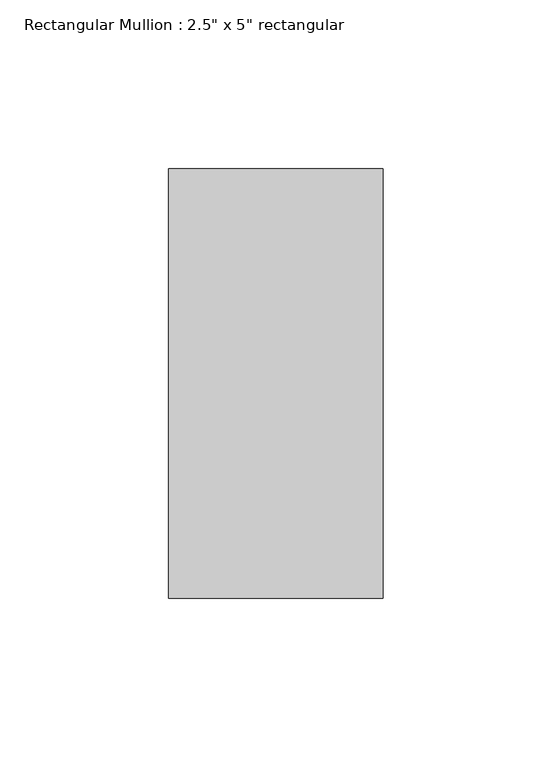
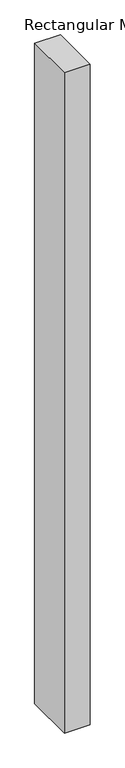
"""IFC4 building model written with IfcOpenShell, lengths in millimetres: member geometry."""

from ifc_helpers import new_model, si_unit, frame, origin, place, context, project, spatial, polyline, outline, extrude, source, transform, mapped, element, save


def member_481990fb(model_context):
    return source(origin(), model_context, "Body", "SweptSolid", [
        extrude(outline(polyline([(31.75, 63.5), (31.75, -63.5), (-31.75, -63.5), (-31.75, 63.5), (31.75, 63.5)])), frame((0.0, 0.0, -1719.9882445), z_axis=(0.0, 0.0, 1.0), x_axis=(1.0, 0.0, 0.0)), (0.0, 0.0, 1.0), 1719.9882445),
    ])


if __name__ == "__main__":
    model = new_model("IFC4")
    model_context = context("Model", 3, world=origin())
    ifc_project = project(units=[si_unit("LENGTHUNIT", "METRE", prefix="MILLI")], contexts=[model_context])
    site = spatial("IfcSite", under=ifc_project)
    building = spatial("IfcBuilding", under=site)
    placement = place(None, origin())
    member_shape = member_481990fb(model_context)
    element("IfcMember", 1, ObjectType="Rectangular Mullion : 2.5\" x 5\" rectangular", at=placement, inside=building, context=model_context, shape_type="MappedRepresentation", body=[
        mapped(member_shape, transform((0.0, 0.0, 0.0), x_axis=(1.0, 0.0, 0.0), y_axis=(0.0, 1.0, 0.0), z_axis=(0.0, 0.0, 1.0))),
    ])
    save(model, "model.ifc")

# Revit data of these elements
# Type "Rectangular Mullion : 2.5\" x 5\" rectangular"
#   built-in parameter 1007304 = 0.416667 (stored number, unit not read)
#   built-in parameter 1007301 = 0.104167 (stored number, unit not read)
#   built-in parameter 1007300 = 0.104167 (stored number, unit not read)
# Element 1 (IfcMember, "Rectangular Mullion : 2.5\" x 5\" rectangular")
#   Materials on its faces: "Aluminum"
# Materials
#   "Aluminum": class "Metal", colour RGB 247 247 247, transparency 0, Description = "Aluminum 6061", Cost = 0
